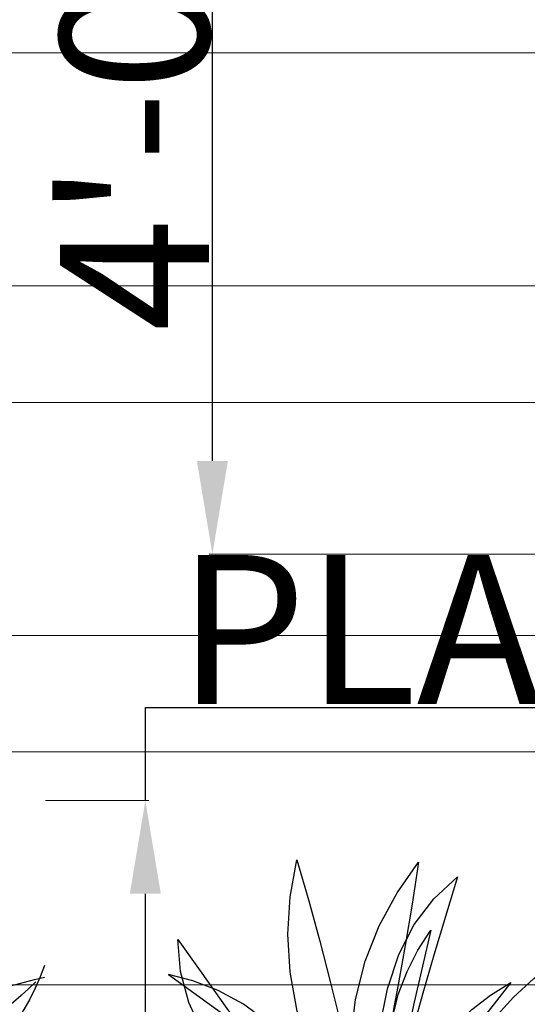
# Model space of a CAD drawing. Units: inches. Extents: x 351 to 1738, y -265 to 286.
# Tile 17 of 38: x 1209 to 1236, y -175 to -122. Entities that reach past the tile are written whole.
import ezdxf

# ---------------------------------------------------------------- set-up
doc = ezdxf.new("R2010")
doc.units = ezdxf.units.IN
doc.header["$MEASUREMENT"] = 0
doc.layers.add('A-ANNO-DIMS', color=2, linetype='Continuous', lineweight=18)
doc.layers.add('A-FLOR-PATT', color=9, linetype='Continuous', lineweight=9)
for name, color, linetype in [('CAY', 94, 'Continuous'), ('CHITIET', 144, 'Continuous'), ('DIENHOA', 3, 'Continuous'), ('netmanh', 9, 'Continuous'), ('VATDUNG', 9, 'Continuous')]:
    doc.layers.add(name, color=color, linetype=linetype)
doc.styles.get("Standard").update_dxf_attribs({"font": 'arial.ttf'})
doc.dimstyles.get("Standard").update_dxf_attribs({"dimtxt": 8, "dimasz": 5, "dimexe": 0.18, "dimexo": 0.0625, "dimgap": 0.09, "dimtad": 1, "dimtoh": 1, "dimzin": 0, "dimdsep": 46, "dimlunit": 4, "dimtxsty": 'Standard', "dimcen": 0, "dimclre": 256, "dimadec": 0, "dimazin": 0, "dimtfac": 1, "dimtofl": 0, "dimtmove": 0, "dimatfit": 3, "dimfxl": 1, "dimtolj": 1, "dimtzin": 0, "dimlwe": -1, "dimarcsym": 0})

# ---------------------------------------------------------------- blocks, each defined once
blk = doc.blocks.new('Cay03_mb')
at = {"layer": 'DIENHOA'}
for p, q in [((118.6, 555.3), (166.2, 599.1)), ((166.2, 599.1), (142.2, 519.4)), ((79.5, 503.7), (118.6, 555.3)), ((142.2, 519.4), (119, 441.7)), ((48.6, 443.6), (79.5, 503.7)), ((25.5, 374.3), (48.6, 443.6)), ((119, 441.7), (96.7, 365.6)), ((-365.2, 390.3), (-414.4, 402.8)), ((-414.4, 402.8), (-240.2, 277.8)), ((-314.9, 371.3), (-365.2, 390.3)), ((-263.5, 343.5), (-314.9, 371.3)), ((9.9, 295.3), (25.5, 374.3)), ((96.7, 365.6), (75.6, 290.6)), ((-211.2, 304.6), (-263.5, 343.5))]:
    blk.add_line(p, q, dxfattribs=at)
for points in [[(23.7, -5.4), (-41, 82.2), (-91.8, 167.1), (-129.7, 249.5), (-155.6, 329.6), (-170.2, 407.8), (-174.7, 484.2), (-169.8, 559.3), (-156.5, 633.1)], [(-156.5, 633.1), (-132.5, 551.3), (-110.5, 470), (-89.8, 389.2), (-69.6, 309), (-49, 229.4), (-27.1, 150.4), (-3.2, 72.1), (23.7, -5.4)], [(-16.4, -26.7), (-38.3, 80), (-48.9, 178.3), (-48.7, 269), (-38.5, 352.6), (-19.1, 429.7), (9, 501), (44.9, 567.1), (87.9, 628.5)], [(87.9, 628.5), (75.5, 544.2), (61.3, 461.2), (46.1, 379.1), (30.8, 297.8), (16.1, 216.9), (2.9, 136), (-8.3, 54.9), (-16.4, -26.7)], [(23.7, -5.4), (19.8, 93), (20.3, 177), (25, 248.5), (34, 309.8), (47.3, 362.7), (64.9, 409.3), (86.8, 451.7), (112.9, 491.9)], [(112.9, 491.9), (96, 419.7), (79.5, 347.4), (63.9, 276.5), (50, 208.4), (38.4, 144.8), (29.7, 86.9), (24.6, 36.3), (23.7, -5.4)], [(-395.6, 473.7), (-347.5, 405.6), (-300.6, 339.5), (-254.3, 275.1), (-208.3, 212.3), (-161.9, 150.9), (-114.8, 90.7), (-66.5, 31.6), (-16.4, -26.7)], [(-16.4, -26.7), (-108.3, 38.6), (-186.9, 101.7), (-252.4, 163.5), (-305.1, 224.4), (-345.4, 285.2), (-373.7, 346.6), (-390.4, 409.2), (-395.6, 473.7)], [(23.7, -5.4), (79.9, 91.7), (134.1, 176.2), (185.8, 248.4), (234.3, 308.7), (279, 357.3), (319.3, 394.8), (354.6, 421.4), (384.3, 437.5)], [(273.2, 387.3), (227.6, 328.8), (182.3, 270.1), (138.4, 212.3), (97.2, 156.4), (60, 103.4), (27.8, 54.6), (1.9, 10.8), (-16.4, -26.7)], [(-16.4, -26.7), (21.4, 64.2), (57, 140.3), (91.4, 203.3), (125.2, 255.1), (159.5, 297.5), (195, 332.5), (232.7, 361.8), (273.2, 387.3)]]:
    blk.add_lwpolyline(points, dxfattribs=at)
blk = doc.blocks.new('A$C5431134F')
at = {"layer": 'VATDUNG'}
for centre, radius, start, end in [((2160.8, 1662), 1245, 150.2411, 205.809), ((5177, 1582.5), 4150.3, 170.24, 186.1148), ((-65.9, 1738.8), 1267.2, 354.3326, 25.2804), ((193.1, 3473.3), 2507.8, 289.6318, 316.9416), ((2357.8, 162.2), 1629.1, 101.2486, 143.9899), ((1000.7, 2213.1), 1133.8, 274.4073, 336.4431), ((1532.8, 1250.1), 499, 101.4267, 190.9877), ((1828.1, 1082.8), 773.2, 121.9055, 175.1859), ((3715.1, 660.2), 2523.5, 154.6853, 162.4501), ((-246.7, 51.1), 1647.5, 39.15, 81.389), ((1000.7, 2213.1), 1133.8, 208.0484, 264.6491), ((1859.5, 3770.4), 2797.6, 228.5745, 252.3842), ((1101.5, 1552.5), 361.2, 169.1166, 218.9556), ((667.9, 1279.8), 349.9, 42.8374, 76.9786), ((-929.9, 388.9), 2082.1, 20.5138, 36.0242), ((1386.4, 1856.4), 738.5, 261.6389, 315.6255), ((-169.9, 6392.7), 5465.7, 286.3355, 292.415), ((1571.2, 1428.8), 356.3, 257.3557, 344.3532), ((624.5, 223.6), 940.4, 92.4374, 115.2956), ((-65.9, 1738.8), 1267.2, 330.7697, 331.9367), ((1294.4, -49.6), 1206.1, 104.1284, 160.1468), ((-2233.8, 3749.8), 4146.2, 305.4464, 320.7382), ((2052.7, 864.5), 1083.3, 166.3603, 232.9474), ((1250.8, 281.5), 836.9, 19.4342, 107.4357), ((625, 349.3), 851.8, 6.5073, 62.3609), ((-70, 1420), 1084.7, 282.2423, 341.7321), ((546.4, 1826.6), 819.5, 246.7315, 287.3971), ((248.9, 8461.8), 7388, 269.91003, 274.50199), ((3885.3, 1488.7), 2894, 188.0959, 210.7226), ((1889.6, 1210.8), 871.9, 188.5552, 241.3289), ((-527.8, -458.7), 2192.5, 24.7599, 44.6473), ((2594.9, 3037.7), 2500, 231.5416, 257.1764), ((754.1, -691.9), 1814.1, 46.1483, 80.3711), ((1738.9, 617.5), 897.6, 155.9893, 202.84), ((2946.5, 414), 2039.9, 165.0604, 184.0737), ((1214.1, 597.8), 452.1, 154.5276, 228.0163), ((-246.7, 51.1), 1647.5, 358.2222, 17.8583)]:
    blk.add_arc(centre, radius, start, end, dxfattribs=at)
blk = doc.blocks.new('A$C5A8625A6')
at = {"layer": 'CHITIET', "ltscale": 50, "xscale": -0.49, "yscale": 0.49, "zscale": 0.49, "rotation": 180}
blk.add_blockref('A$C5431134F', (0, 1120.2), dxfattribs=at)
blk = doc.blocks.new('A$C18571848')
at = {"layer": 'netmanh', "xscale": 0.5393606399999998, "yscale": 0.5393606399999998, "zscale": 0.5393606399999998}
blk.add_blockref('A$C5A8625A6', (0, 0), dxfattribs=at)
blk = doc.blocks.new('*D36')
at = {"layer": 'A-ANNO-DIMS', "transparency": 16777216}
for p, q in [((1073.569, -199.341), (1073.569, -204.202)), ((1105.198, -199.341), (1105.198, -204.202))]:
    blk.add_line(p, q, dxfattribs=at)
at = {"layer": 'A-ANNO-DIMS', "color": 0, "lineweight": -2, "transparency": 16777216}
for p, q in [((1078.569, -204.022), (1100.198, -204.022)), ((1105.198, -204.022), (1227.071, -204.022))]:
    blk.add_line(p, q, dxfattribs=at)
at = {"layer": 'A-ANNO-DIMS', "color": 0, "transparency": 16777216}
for points in [[(1078.569, -203.189), (1078.569, -204.856), (1073.569, -204.022)], [(1100.198, -203.189), (1100.198, -204.856), (1105.198, -204.022)]]:
    blk.add_solid(points, dxfattribs=at)
at = {"layer": 'Defpoints', "color": 0, "transparency": 16777216}
for p in [(1073.569, -199.278), (1105.198, -199.278), (1105.198, -204.022)]:
    blk.add_point(p, dxfattribs=at)
at = {"layer": 'A-ANNO-DIMS', "color": 0, "transparency": 16777216, "insert": (1168.634, -199.796), "char_height": 8, "attachment_point": 5}
blk.add_mtext('\\A1;PLANT A 2\'-7 1/2" TYP.', dxfattribs=at)
blk = doc.blocks.new('*D38')
at = {"layer": 'A-ANNO-DIMS', "color": 0, "lineweight": -2, "transparency": 16777216}
for p, q in [((1215.465, -164.135), (1215.465, -159.135)), ((1215.465, -159.135), (1313.607, -159.135)), ((1215.465, -195.235), (1215.465, -169.135))]:
    blk.add_line(p, q, dxfattribs=at)
at = {"layer": 'A-ANNO-DIMS', "transparency": 16777216}
for p, q in [((1210.112, -164.135), (1215.645, -164.135)), ((1210.112, -200.235), (1215.645, -200.235))]:
    blk.add_line(p, q, dxfattribs=at)
at = {"layer": 'A-ANNO-DIMS', "color": 0, "transparency": 16777216}
for points in [[(1214.631, -169.135), (1216.298, -169.135), (1215.465, -164.135)], [(1214.631, -195.235), (1216.298, -195.235), (1215.465, -200.235)]]:
    blk.add_solid(points, dxfattribs=at)
at = {"layer": 'Defpoints', "color": 0, "transparency": 16777216}
for p in [(1210.05, -164.135), (1215.465, -164.135), (1210.05, -200.235)]:
    blk.add_point(p, dxfattribs=at)
at = {"layer": 'A-ANNO-DIMS', "color": 0, "transparency": 16777216, "insert": (1264.581, -154.958), "char_height": 8, "attachment_point": 5}
blk.add_mtext('\\A1;PLANT B 3\'-0" TYP.', dxfattribs=at)
blk = doc.blocks.new('*D65')
at = {"layer": 'A-ANNO-DIMS', "transparency": 16777216}
for p, q in [((1248.45, -102.915), (1218.882, -102.915)), ((1248.45, -150.915), (1218.882, -150.915))]:
    blk.add_line(p, q, dxfattribs=at)
at = {"layer": 'A-ANNO-DIMS', "color": 0, "lineweight": -2, "transparency": 16777216}
blk.add_line((1219.062, -145.915), (1219.062, -107.915), dxfattribs=at)
at = {"layer": 'A-ANNO-DIMS', "color": 0, "transparency": 16777216}
for points in [[(1218.229, -107.915), (1219.896, -107.915), (1219.062, -102.915)], [(1218.229, -145.915), (1219.896, -145.915), (1219.062, -150.915)]]:
    blk.add_solid(points, dxfattribs=at)
at = {"layer": 'Defpoints', "color": 0, "transparency": 16777216}
for p in [(1219.062, -102.915), (1248.512, -102.915), (1248.512, -150.915)]:
    blk.add_point(p, dxfattribs=at)
at = {"layer": 'A-ANNO-DIMS', "color": 0, "transparency": 16777216, "insert": (1214.888, -126.915), "char_height": 8, "attachment_point": 5, "rotation": 90}
blk.add_mtext('\\A1;4\'-0"', dxfattribs=at)

msp = doc.modelspace()

# ---------------------------------------------------------------- hatches: boundary and pattern name
at = {"layer": 'A-FLOR-PATT', "transparency": 33554559}
h = msp.add_hatch(dxfattribs=at)
h.set_pattern_fill('ANSI37', color=256, scale=200, angle=135)
h.set_pattern_definition([(180, (1112.704, -164.037), (-2e-15, -25), []), (270, (1112.704, -164.037), (25, -5e-15), [])])
h.paths.add_polyline_path([(1380.064, 73.463), (1380.132, 148.463), (1338.064, 148.463), (1290.704, 148.463), (1290.704, 88.463), (1248.704, 88.463), (1248.704, -2.009), (1244.704, -2.009), (1244.704, 142.457), (1160.704, 142.457), (1160.704, 158.963), (1160.704, 170.137), (1160.704, 206.137), (1160.704, 228.963), (1112.704, 228.963), (1112.704, 209.963), (1112.704, 168.963), (1124.704, 168.963), (1124.704, 162.963), (1112.704, 162.963), (1112.704, 64.463), (1112.704, 60.463), (1112.704, 0.463), (1112.704, -48.026), (1146.804, -47.981), (1146.804, -35.691), (1207.804, -35.691), (1207.804, -47.902), (1236.542, -47.864), (1236.544, -50.009), (1248.5, -50.009), (1248.506, -102.915), (1248.512, -150.915), (1248.514, -164.037), (1248.549, -164.037), (1273.017, -164.037), (1273.017, -128.799), (1355.24, -128.799), (1355.24, -164.037), (1384.204, -164.037), (1384.204, -57.037), (1380.064, -57.037), (1380.064, -48.037), (1392.064, -48.037), (1392.064, -53.037), (1406.549, -53.037), (1406.549, -57.037), (1401.204, -57.037), (1401.204, -147.037), (1468.204, -147.037), (1468.204, -138.5), (1472.204, -138.5), (1472.204, -102.5), (1468.204, -102.5), (1468.204, -57.037), (1442.549, -57.037), (1442.549, -53.037), (1463.049, -53.037), (1463.049, -40.747), (1524.049, -40.747), (1524.049, -48.037), (1536.064, -48.037), (1536.064, -53.037), (1557.704, -53.037), (1557.704, 204.963), (1384.204, 204.963), (1384.204, 73.463), (1392.064, 73.463), (1392.064, 64.463), (1384.204, 64.463), (1384.204, -3.5), (1380.204, -3.537), (1380.204, 64.463), (1380.064, 64.463)])
h.paths.add_polyline_path([(1510.714, 86.458, -0.103984), (1511.661, 85.595, 0.470438), (1510.158, 87.614, 0.0961)], flags=16)
h.paths.add_polyline_path([(1510.443, 100.266, 0.009798), (1504.693, 100.48, 0.02879), (1504.6, 99.767, -0.165331), (1505.519, 96.135, -0.143601)], flags=16)
h.paths.add_polyline_path([(1487.201, 85.595, -0.103984), (1488.148, 86.458, 0.0961), (1488.704, 87.614, 0.470438)], flags=0)
h.paths.add_polyline_path([(1495.052, 100.43), (1494.178, 100.43, -0.026463), (1494.262, 99.774, -0.144219)], flags=16)
h.paths.add_polyline_path([(1444.485, 86.458, -0.103984), (1445.433, 85.595, 0.470438), (1443.93, 87.614, 0.0961)], flags=16)
h.paths.add_polyline_path([(1420.972, 85.595, -0.103984), (1421.92, 86.458, 0.0961), (1422.475, 87.614, 0.470438)], flags=16)
h.paths.add_polyline_path([(1428.632, 100.335, 0.001054), (1427.971, 100.309, -0.021524), (1428.033, 99.774, -0.114301)], flags=16)
h.paths.add_polyline_path([(1419.906, 143.708, 0.024979), (1420.222, 157.526), (1421.573, 159.101), (1421.573, 175.369), (1391.393, 175.369), (1391.393, 200.519), (1542.294, 200.519), (1542.294, 175.369), (1512.028, 175.369, 0.019865), (1511.521, 153.838, 0.025134), (1512.758, 118.323, 0.020553), (1512.942, 115.253), (1419.834, 115.253, -0.000414), (1419.843, 124.798), (1413.059, 124.798), (1413.059, 84.437, -0.061853), (1415.831, 80.45, -0.093077), (1420.972, 85.595, -0.267537), (1422.371, 84.732, 0.08511), (1424.052, 84.616, -0.885393), (1424.033, 84.851, -1.125815), (1424.073, 84.366, -0.087987), (1422.371, 84.732, -0.267537), (1422.326, 83.089, -0.370542), (1420.972, 85.595, 0.093077), (1415.831, 80.45, -0.087414), (1417.914, 73.937), (1418.941, 73.937, 0.02725), (1418.913, 76.906, -0.115703), (1421.051, 73.937), (1445.354, 73.937, -0.115703), (1447.492, 76.906, 0.02725), (1447.464, 73.937), (1448.491, 73.937, -0.087414), (1450.574, 80.45, 0.093077), (1445.433, 85.595, -0.370542), (1444.079, 83.089, -0.267537), (1444.034, 84.732, -0.087987), (1442.332, 84.366, -1.125815), (1442.372, 84.851, -2.032736), (1442.364, 84.368, 0.086378), (1444.034, 84.732, -0.267537), (1445.433, 85.595, -0.093077), (1450.574, 80.45, -0.257732), (1466.483, 90.927, -0.47867), (1468.832, 91.907, -0.47867), (1471.18, 90.927, -0.26264), (1483.053, 81.78, -0.071866), (1487.201, 85.595, -0.267537), (1488.6, 84.732, 0.08511), (1490.28, 84.616, -0.885393), (1490.262, 84.851, -1.125815), (1490.301, 84.366, -0.087987), (1488.6, 84.732, -0.267537), (1488.554, 83.089, -0.370542), (1487.201, 85.595, 0.071866), (1483.053, 81.78, -0.132065), (1484.143, 73.937), (1485.169, 73.937, 0.02725), (1485.142, 76.906, -0.115703), (1487.28, 73.937), (1511.582, 73.937, -0.115703), (1513.72, 76.906, 0.02725), (1513.693, 73.937), (1514.719, 73.937, -0.087414), (1516.802, 80.45, 0.093077), (1511.661, 85.595, -0.370542), (1510.308, 83.089, -0.267537), (1510.262, 84.732, -0.087987), (1508.561, 84.366, -1.125815), (1508.601, 84.851, -2.032736), (1508.592, 84.368, 0.086378), (1510.262, 84.732, -0.267537), (1511.661, 85.595, -0.093077), (1516.802, 80.45, -0.061853), (1519.575, 84.437), (1519.575, 73.937), (1413.059, 73.937), (1413.059, 124.798), (1419.843, 124.798, -0.000821)], flags=16)
h.paths.add_polyline_path([(1220.149, 54.133, -0.103984), (1220.869, 53.476, 0.470438), (1219.727, 55.011, 0.0961)], flags=16)
h.paths.add_polyline_path([(1219.944, 64.626, 0.009798), (1215.574, 64.789, 0.02879), (1215.503, 64.247, -0.165331), (1216.201, 61.487, -0.143601)], flags=16)
h.paths.add_polyline_path([(1209.779, 64.449, 0.097446), (1209.339, 64.751), (1208.247, 64.751, 0.12739), (1207.7, 64.326, 0.171586), (1206.95, 61.475, -0.158854), (1207.636, 59.45, 0.015898), (1207.795, 59.218, 0.061546), (1208.598, 59.616, 0.175416), (1208.638, 60.099, -0.284779), (1209.348, 62.472, 0.326216)], flags=16)
h.paths.add_polyline_path([(1169.818, 54.133, -0.103984), (1170.538, 53.476, 0.470438), (1169.396, 55.011, 0.0961)], flags=16)
h.paths.add_polyline_path([(1159.017, 62.472, 0.284764), (1158.307, 60.099, -0.175433), (1158.267, 59.616, 0.39293), (1159.448, 64.449, -0.32623)], flags=16)
h.paths.add_polyline_path([(1156.342, 58.239, -0.178321), (1154.011, 55.31, -0.174736), (1154.722, 55.233, -0.200802), (1156.27, 56.086, 0.12699), (1157.283, 58.991, -0.091205)], flags=16)
h.paths.add_polyline_path([(1156.624, 61.413, 0.157275), (1157.316, 64.247, 0.169622)], flags=16)
h.paths.add_polyline_path([(1152.67, 54.133, -0.0961), (1151.95, 53.476, 0.064076), (1154.465, 54.384, 0.199016)], flags=16)
h.paths.add_polyline_path([(1202.281, 53.476, -0.103984), (1203, 54.133, 0.0961), (1203.423, 55.011, 0.470438)], flags=0)
h.paths.add_polyline_path([(1151.139, 97.64, 0.024979), (1151.379, 108.141), (1152.406, 109.338), (1152.406, 121.701), (1129.47, 121.701), (1129.47, 140.814), (1244.149, 140.814), (1244.149, 121.701), (1221.148, 121.701, 0.019865), (1220.763, 105.338, 0.025134), (1221.703, 78.349, 0.020553), (1221.843, 76.016), (1151.078, 76.016, -0.128743), (1148.786, 65.037, 0.539352), (1150.327, 64.171, -0.027594), (1163.481, 64.751, 0.097695), (1163.04, 64.449, 0.326216), (1163.471, 62.472, -0.284777), (1164.181, 60.099, -0.194757), (1165.846, 61.443, -0.155402), (1165.172, 64.247, -0.166022), (1165.869, 61.475, -0.177014), (1167.852, 62.77, -0.448203), (1169.974, 60.807, -0.393499), (1167.679, 57.86, -0.895548), (1168.438, 54.524, -0.355767), (1166.218, 56.086, -0.066024), (1165.505, 57.539), (1165.251, 56.243, -0.371732), (1164.02, 59.758, -0.373614), (1163.04, 64.449, -0.097695), (1163.481, 64.751, 0.021354), (1153.294, 64.429, -0.134183), (1156.695, 61.368, 0.186873), (1154.636, 62.77, 0.448203), (1152.514, 60.807, 0.403726), (1154.905, 57.846, 0.711219), (1153.334, 55, 0.53154), (1151.95, 53.476, -0.267537), (1153.013, 52.821, 0.08511), (1154.29, 52.732, -0.885393), (1154.276, 52.911, -1.125815), (1154.306, 52.543, -0.087987), (1153.013, 52.821, -0.267537), (1152.978, 51.572, -0.370542), (1151.95, 53.476, 0.093077), (1148.043, 49.566, -0.087414), (1149.626, 44.617), (1150.406, 44.617, 0.02725), (1150.385, 46.873, -0.115703), (1152.01, 44.617), (1170.478, 44.617, -0.115703), (1172.103, 46.873, 0.02725), (1172.082, 44.617), (1172.862, 44.617, -0.087414), (1174.445, 49.566, 0.093077), (1170.538, 53.476, -0.370542), (1169.51, 51.572, -0.267537), (1169.475, 52.821, -0.087987), (1168.182, 52.543, -1.125815), (1168.212, 52.911, -2.032736), (1168.206, 52.544, 0.086378), (1169.475, 52.821, -0.267537), (1170.538, 53.476, -0.093077), (1174.445, 49.566, -0.257732), (1186.536, 57.528, -0.47867), (1188.321, 58.273, -0.47867), (1190.106, 57.528, -0.26264), (1199.128, 50.577, -0.071866), (1202.281, 53.476, -0.267537), (1203.344, 52.821, 0.08511), (1204.621, 52.732, -0.885393), (1204.607, 52.911, -1.125815), (1204.637, 52.543, -0.087987), (1203.344, 52.821, -0.267537), (1203.309, 51.572, -0.370542), (1202.281, 53.476, 0.071866), (1199.128, 50.577, -0.132065), (1199.957, 44.617), (1200.737, 44.617, 0.02725), (1200.716, 46.873, -0.115703), (1202.341, 44.617), (1220.809, 44.617, -0.115703), (1222.434, 46.873, 0.02725), (1222.413, 44.617), (1223.193, 44.617, -0.087414), (1224.776, 49.566, 0.093077), (1220.869, 53.476, -0.370542), (1219.841, 51.572, -0.267537), (1219.806, 52.821, -0.087987), (1218.513, 52.543, -1.125815), (1218.543, 52.911, -2.032736), (1218.537, 52.544, 0.086378), (1219.806, 52.821, -0.267537), (1220.869, 53.476, -0.093077), (1224.776, 49.566, -0.061853), (1226.883, 52.597), (1226.883, 44.617), (1145.936, 44.617), (1145.936, 83.269), (1151.091, 83.269, -0.000821)], flags=16)
h.paths.add_polyline_path([(1218.01, 57.86, -0.895548), (1218.769, 54.524, -0.355767), (1216.549, 56.086, -0.066024), (1215.836, 57.539), (1215.582, 56.243, -0.371732), (1214.351, 59.758, -0.373614), (1213.371, 64.449, 0.326216), (1213.802, 62.472, -0.284777), (1214.512, 60.099, -0.194757), (1216.177, 61.443, -0.179991), (1218.183, 62.77, -0.448203), (1220.305, 60.807, -0.393499)], flags=16)
h.paths.add_polyline_path([(1424.735, 91.363, -0.393499), (1421.715, 95.241, -0.448203), (1424.507, 97.824, -0.179991), (1427.147, 96.077, -0.194757), (1429.338, 94.309, -0.284777), (1430.272, 97.432, 0.326216), (1430.839, 100.034, -0.373614), (1429.55, 93.861, -0.371732), (1427.929, 89.235), (1427.596, 90.941, -0.066024), (1426.657, 89.029, -0.355767), (1423.736, 86.973, -0.895548)], flags=16)
h.paths.add_polyline_path([(1238.033, 131.257, -1), (1227.329, 131.257, -1)], flags=0)
h.paths.add_polyline_path([(1235.357, 131.257, -1), (1230.005, 131.257, -1)], flags=0)
h.paths.add_polyline_path([(1214.039, 54.243, 0.154382), (1214.38, 53.992, 0.358955), (1213.613, 54.016, 0.603948), (1214.379, 53.657, 0.371319), (1213.968, 52.872, 0.187994), (1214.312, 52.809, -0.592455), (1213.953, 52.967, -0.294279), (1214.083, 53.691, -1.300187), (1213.881, 54.134, -0.283762), (1214.469, 53.896, 1.15094)], flags=16)
h.paths.add_polyline_path([(1212.091, 56.286, -0.408434), (1211.337, 56.445, -0.036259), (1211.098, 56.848, -0.236098), (1211.59, 56.63, 0.035345), (1211.835, 56.543, -0.475241), (1212.091, 56.286, -0.475241), (1212.438, 56.182, 0.035345), (1212.631, 56.007, -0.236098), (1213.056, 55.676, -0.036259), (1212.588, 55.697, -0.408434)], flags=16)
h.paths.add_polyline_path([(1211.469, 50.297, 0.296043), (1210.47, 50.527, 0.310883), (1211.931, 50.148, 0.021255)], flags=16)
h.paths.add_polyline_path([(1213.739, 51.818, -0.036259), (1213.271, 51.838, -0.408434), (1212.774, 52.427, -0.094786), (1212.293, 50.703, 1.150474), (1212.911, 50.232, 0.166288), (1213.265, 50.68, -0.025254), (1212.603, 50.13, 1.087932), (1212.471, 49.407, 0.166288), (1213.02, 49.251, -0.016128), (1212.567, 49.563, -0.286859), (1212.217, 49.638, 0.022156), (1212.046, 50.055, -0.64613), (1212.185, 50.498, 0.088412), (1212.732, 52.077, -1.186037), (1213.121, 52.323, 0.035345), (1213.314, 52.148, -0.236098)], flags=16)
h.paths.add_polyline_path([(1212.094, 50.342, -0.048524), (1211.54, 49.605, -1.103834), (1211.397, 48.738, -0.785515), (1211.683, 48.254, -0.392043), (1210.948, 48.525, -0.392819), (1210.561, 47.995, -0.592455), (1210.201, 48.153, -0.294279), (1210.331, 48.877, -0.704172), (1210.316, 49.592, -0.679344), (1210.729, 50.112, 0.563676)], flags=16)
h.paths.add_polyline_path([(1211.274, 49.829, -0.139826), (1210.745, 49.859, -0.217879), (1210.948, 49.509, -0.498572)], flags=0)
h.paths.add_polyline_path([(1433.426, 81.49, -0.181571), (1434.245, 81.788, -0.008067), (1433.726, 82.205, 0.045578), (1432.755, 81.242, 0.179011)], flags=16)
h.paths.add_polyline_path([(1434.146, 81.009, -0.132442), (1433.645, 80.771, 0.259089), (1433.234, 80.471, -0.180211), (1433.392, 80.805, -0.16994), (1432.758, 81.109, 0.032652), (1433.273, 80.474, -0.493363), (1434.046, 80.146, -0.390497)], flags=16)
h.paths.add_polyline_path([(1434.83, 80.047, -0.947538), (1435.294, 79.576, -0.299128), (1434.625, 79.404, -0.270439), (1435.01, 78.591, -0.592455), (1434.537, 78.382, -0.392819), (1434.027, 79.08, -0.392043), (1433.06, 78.723, -0.352042), (1433.003, 79.197, -0.197216), (1433.75, 79.734, -0.71364), (1434.447, 79.939, -0.21479), (1434.819, 80.475, 0.408833), (1435.075, 80.803, -0.226152)], flags=16)
h.paths.add_polyline_path([(1432.67, 81.217, -0.454218), (1431.897, 79.923, -0.414411), (1431.301, 80.035, 0.016129), (1431.897, 80.445, 0.27957), (1432.073, 80.871, -0.289504), (1431.103, 81.321, -0.414411), (1430.978, 81.915, 0.01613), (1431.586, 81.521, 0.341293), (1432.125, 81.583, -0.813186)], flags=16)
h.paths.add_polyline_path([(1429.893, 86.381, -0.947538), (1430.358, 85.91, -0.173106), (1429.984, 85.712, -0.038817), (1431.625, 84.214, -0.0879), (1432.097, 88.549, -0.049768), (1431.254, 88.49, -0.236098), (1431.814, 88.925, 0.035345), (1432.067, 89.155, -0.475241), (1432.524, 89.291, -0.475241), (1432.86, 89.63, 0.035345), (1433.182, 89.744, -0.236098), (1433.83, 90.032, -0.036259), (1433.516, 89.502, -0.408434), (1432.524, 89.291, -0.312424), (1432.106, 88.58, 0.088559), (1431.625, 84.214, -0.408434), (1430.971, 83.439, -0.036259), (1430.355, 83.412, -0.236098), (1430.914, 83.847, 0.035345), (1431.168, 84.078, -0.475241), (1431.625, 84.214, 0.038817), (1429.984, 85.712, -0.321732), (1429.333, 86.048, -0.32743), (1429.883, 86.809, 0.408833), (1430.138, 87.138, -0.226152)], flags=16)
h.paths.add_polyline_path([(1211.206, 58.616, -0.999784), (1211.336, 59.323, -0.614994)], flags=16)
h.paths.add_polyline_path([(1210.288, 49.429, 0.154382), (1210.629, 49.178, 0.358955), (1209.861, 49.202, 0.603948), (1210.627, 48.843, -0.534825), (1210.806, 49.295, 0.748346)], flags=16)
h.paths.add_polyline_path([(1209.589, 51.828, -0.008791), (1209.775, 51.753, 0.112231), (1209.466, 52.019, 1.418851), (1209.014, 51.708, -0.458726), (1208.651, 51.073, -0.592455), (1208.291, 51.232, -0.294279), (1208.421, 51.955, -1.300187), (1208.219, 52.398, -0.226005), (1208.719, 52.257, -0.475519), (1209.158, 52.369, -1.455499), (1209.603, 52.664, 0.421305), (1209.191, 52.262, -0.591212), (1208.979, 51.796, 0.497399), (1209.773, 51.333, 0.649312)], flags=16)
h.paths.add_polyline_path([(1208.029, 52.041, 0.544667), (1208.832, 52.045, 0.220132)], flags=0)
h.paths.add_polyline_path([(1210.438, 51.425, -0.2042), (1210.277, 52.018, 0.270826), (1209.915, 52.897, 0.324115)], flags=0)
h.paths.add_polyline_path([(1209.668, 52.407, -0.60139), (1208.99, 52.221, -0.394916), (1208.248, 52.83, -0.836792), (1208.651, 53.017, -0.338488), (1209.039, 52.571, 0.194138), (1209.191, 52.262, 0.413995), (1209.712, 52.475, 0.51771), (1210.503, 51.416, 0.401922), (1209.493, 50.93, 0.206396), (1209.516, 50.165, -0.319463), (1210.417, 51.418, -0.466635)], flags=16)
h.paths.add_polyline_path([(1206.601, 56.086, -0.355767), (1204.381, 54.524, -0.921198), (1205.236, 57.846, 0.206569), (1207.614, 58.991, -0.12699)], flags=16)
h.paths.add_polyline_path([(1435.487, 82.816, 0.527765), (1436.615, 83.361, 0.50854), (1437.05, 82.433, 0.592455), (1437.524, 82.641, 0.331245), (1436.963, 83.548, 0.387863), (1437.808, 83.626, 0.592954), (1437.618, 84.176, 0.226016), (1436.961, 83.99, 0.318205), (1437.588, 84.854, 0.689374), (1437.05, 84.991, 0.335765), (1436.539, 84.41, -0.156993), (1436.404, 84.065, -0.434611), (1436.961, 83.99, -0.21479), (1437.333, 84.526, 0.408833), (1437.588, 84.854, -0.226152), (1437.343, 84.097, -0.947538), (1437.808, 83.626, -0.299128), (1437.139, 83.455, -0.270439), (1437.524, 82.641, -0.592455), (1437.05, 82.433, -0.392819), (1436.541, 83.13, -0.43966), (1435.475, 82.794, -0.174614), (1435.942, 82.244, -0.206396), (1435.912, 81.237, -0.270826), (1435.125, 82.208, 0.207976), (1434.686, 82.904, -0.196495)], flags=16)
h.paths.add_polyline_path([(1435.386, 84.832, 0.270811), (1434.91, 83.676, -0.204217), (1434.699, 82.895, 0.324115)], flags=0)
h.paths.add_polyline_path([(1435.68, 84.18, -0.217656), (1435.554, 83.304, -0.176705), (1436.236, 83.778, -0.373036)], flags=0)
h.paths.add_polyline_path([(1435.566, 100.034, 0.326216), (1436.133, 97.432, -0.284777), (1437.067, 94.309, -0.194757), (1439.258, 96.077, -0.155402), (1438.371, 99.767, -0.166022), (1439.289, 96.12, -0.177014), (1441.897, 97.824, -0.448203), (1444.69, 95.241, -0.393499), (1441.67, 91.363, -0.895548), (1442.669, 86.973, -0.355767), (1439.748, 89.029, -0.066024), (1438.809, 90.941), (1438.476, 89.235, -0.371732), (1436.855, 93.861, -0.373614)], flags=16)
h.paths.add_polyline_path([(1191.252, 49.507, -0.274022), (1190.658, 48.409, 0.267537), (1191.311, 47.344, 0.370542)], flags=0)
h.paths.add_polyline_path([(1190.301, 49.717, 0.199016), (1188.619, 49.04, 0.064076), (1191.252, 49.507, -0.0961)], flags=0)
h.paths.add_polyline_path([(1189.518, 47.857, 1.125815), (1189.676, 47.523, 2.044605)], flags=0)
h.paths.add_polyline_path([(1464.974, 80.372, 0.274022), (1465.756, 78.927, -0.083013)], flags=0)
h.paths.add_polyline_path([(1464.974, 80.372, 0.370542), (1464.897, 77.525, 0.576324)], flags=0)
h.paths.add_polyline_path([(1464.974, 80.372, -0.470438), (1467.284, 81.372, -0.0961), (1466.226, 80.648, -0.199016), (1468.439, 79.757, -0.064076)], flags=0)
h.paths.add_polyline_path([(1189.511, 56.43, -0.259467), (1188.321, 56.391, -0.259467), (1187.13, 56.43, 0.08511), (1188.193, 55.716, -0.885393), (1188.27, 55.878, -1.196013), (1188.355, 55.442, 0.101459)], flags=0)
h.paths.add_polyline_path([(1188.321, 57.596, 0.078072), (1187.678, 57.24, 0.01555), (1188.321, 57.136, 0.01555), (1188.964, 57.24, 0.078072)], flags=0)
h.paths.add_polyline_path([(1190.164, 55.365, -0.576324), (1190.106, 57.528, -0.198294), (1188.321, 58.319, -0.198294), (1186.536, 57.528, -0.576324), (1186.477, 55.365, -0.370542), (1186.536, 57.528, 0.198294), (1188.321, 58.319, 0.198294), (1190.106, 57.528, -0.370542)], flags=0)
h.paths.add_polyline_path([(1188.372, 55.878, 1.125814), (1188.529, 55.544, 2.044605)], flags=0)
h.paths.add_polyline_path([(1186.341, 49.717, -0.0961), (1185.389, 49.507, 0.064076), (1188.022, 49.04, 0.199016)], flags=0)
h.paths.add_polyline_path([(1185.389, 49.507, -0.267537), (1185.984, 48.409, 0.08511), (1187.046, 47.695, -0.885393), (1187.123, 47.857, -1.125815), (1186.966, 47.523, -0.087987), (1185.984, 48.409, -0.267537), (1185.331, 47.344, -0.370542)], flags=0)
h.paths.add_polyline_path([(1399.441, 187.944, -1), (1413.525, 187.944, -1)], flags=0)
h.paths.add_polyline_path([(1402.962, 187.944, -1), (1410.004, 187.944, -1)], flags=0)
h.paths.add_polyline_path([(1357.663, -72.245), (1377.272, -72.245), (1377.272, -91.854), (1357.663, -91.854)], flags=16)
h.paths.add_polyline_path([(1467.256, 78.201, -1.125815), (1467.049, 77.761, -2.044605)], flags=0)
h.paths.add_polyline_path([(1468.822, 88.714, 0.941125), (1469.106, 88.316, 1.137152), (1468.765, 88.755, 0.890986), (1468.99, 88.245, 0.094828), (1470.398, 89.481, -0.267537), (1471.18, 90.927, -0.028123), (1469.678, 90.547, -0.028774), (1469.948, 90.311, -0.020327), (1468.832, 90.41, -0.020327), (1467.716, 90.311, -0.028774), (1467.986, 90.547, -0.028123), (1466.483, 90.927, -0.267537), (1467.265, 89.481, 0.08511), (1468.663, 88.542, -1.202316)], flags=0)
h.paths.add_polyline_path([(1178.25, 124.523, -0.119929), (1165.65, 124.145, -0.107349), (1159.133, 124.446, -0.102891), (1159.132, 130.465, -0.074897), (1158.993, 137.956, 0.002027), (1167.844, 137.479, -0.07553), (1180.337, 137.666, -0.075861), (1186.502, 137.688, -0.14099), (1186.272, 130.046, -0.095481), (1186.729, 124.748, -0.10603)], flags=0)
h.paths.add_polyline_path([(1469.225, 79.757, -0.199016), (1471.437, 80.648, -0.0961), (1470.379, 81.372, -0.470438), (1472.689, 80.372, -0.370542), (1472.766, 77.525, -0.267537), (1471.907, 78.927, -0.087986), (1470.615, 77.761, -1.125849), (1470.408, 78.201, -2.032736), (1470.642, 77.778, 0.086378), (1471.907, 78.927, -0.267537), (1472.689, 80.372, -0.064076)], flags=0)
h.paths.add_polyline_path([(1430.423, 186.902, -0.074897), (1430.24, 196.758, 0.002027), (1441.887, 196.131, -0.07553), (1458.326, 196.377, -0.075861), (1466.438, 196.406, -0.14099), (1466.136, 186.35, -0.095481), (1466.737, 179.378, -0.10603), (1455.58, 179.082, -0.119929), (1439, 178.585, -0.107349), (1430.425, 178.981, -0.102891)], flags=0)
h.paths.add_polyline_path([(1162.258, 49.939, 0.335765), (1161.87, 49.497, -0.156994), (1161.767, 49.235, -0.434611), (1162.19, 49.178, -0.21479), (1162.473, 49.585, 1.529195)], flags=16)
h.paths.add_polyline_path([(1161.683, 49.021, 0.581518), (1161.268, 49.583, 0.592761)], flags=16)
h.paths.add_polyline_path([(1162.602, 48.058, 0.371319), (1162.192, 48.843, 0.434533), (1162.88, 48.962, 0.185081), (1162.197, 48.926, 1.121837)], flags=16)
h.paths.add_polyline_path([(1161.443, 48.941, -1.307104), (1161.495, 48.571, -0.217752), (1161.136, 48.254, 0.697303), (1161.871, 49.048, 0.121514)], flags=16)
h.paths.add_polyline_path([(1162.531, 49.429, -0.207084), (1162.05, 49.146, -0.99203)], flags=16)
h.paths.add_polyline_path([(1161.304, 49.578, -0.719667), (1161.513, 50.079, -0.130428), (1160.836, 50.168, 0.039593)], flags=0)
h.paths.add_polyline_path([(1162.036, 50.584, -0.008067), (1161.642, 50.9, 0.029367), (1161.35, 50.297, -0.205788)], flags=16)
h.paths.add_polyline_path([(1162.882, 51.392, -0.124733), (1162.763, 51.828, -0.101191), (1162.399, 51.438, -0.153425)], flags=0)
h.paths.add_polyline_path([(1164.235, 51.85, -0.309107), (1164.513, 51.136, -0.627125), (1163.781, 51.603, -0.685909), (1162.777, 51.219, -0.233285), (1163.303, 50.165, -0.270826), (1162.705, 50.903, 0.2042), (1162.381, 51.425, 0.204182), (1162.542, 52.018, -0.270841), (1162.903, 52.897, -0.127261), (1163.219, 52.529, -1.168681), (1163.781, 52.587, -0.329112), (1164.168, 53.017, -0.836792), (1164.571, 52.83, -0.193341), (1164.391, 52.338, -0.947538), (1164.744, 51.981, -0.299128)], flags=16)
h.paths.add_polyline_path([(1163.598, 51.937, -1.262956), (1163.236, 51.831, 0.012575), (1162.971, 51.721, 0.230657), (1163.151, 52.407, -0.164898), (1163.178, 52.661, -0.44932), (1163.628, 52.262, -0.721477), (1164.154, 52.088, -0.849998)], flags=0)
h.paths.add_polyline_path([(1161.613, 58.616, -0.980413), (1161.525, 59.049, -2.908935)], flags=16)
h.paths.add_polyline_path([(1160.252, 49.166, -0.414411), (1159.799, 49.251, 0.016129), (1160.252, 49.563, 0.27957), (1160.386, 49.887, -0.289504), (1159.649, 50.229, -0.414411), (1159.554, 50.68, 0.01613), (1160.015, 50.381, 0.617885), (1160.526, 50.703, -0.094786), (1160.045, 52.427, -0.140444), (1159.682, 52.042, -0.057856), (1159.3, 51.872, 0.544843), (1160.046, 52.419, -0.088122), (1160.404, 55.721, -0.049768), (1159.763, 55.676, -0.236098), (1160.188, 56.007, 0.035345), (1160.381, 56.182, -0.475241), (1160.728, 56.286, -0.475241), (1160.984, 56.543, 0.035345), (1161.229, 56.63, -0.236098), (1161.721, 56.848, -0.036259), (1161.482, 56.445, -0.408434), (1160.728, 56.286, -0.312424), (1160.411, 55.745, 0.088559), (1160.045, 52.427, 0.107081), (1160.634, 50.498, -0.494798), (1160.839, 50.149, -0.454218)], flags=16)
h.paths.add_polyline_path([(1160.666, 49.808, -2.076528), (1160.828, 50.172, 0.019586)], flags=0)
h.paths.add_polyline_path([(1158.439, 53.992, 0.154382), (1158.78, 54.243, 0.748346), (1158.262, 54.109, -0.338225), (1158.492, 53.839, -0.170816), (1159.124, 53.779, 0.495729), (1158.938, 54.134, 0.226016)], flags=16)
h.paths.add_polyline_path([(1160.045, 52.427, 0.038817), (1158.798, 53.565, -0.119818), (1158.574, 53.586, -0.309107), (1158.851, 52.872, -0.187994), (1158.506, 52.809, 0.592455), (1158.866, 52.967, 0.331245), (1158.44, 53.657, 0.201245), (1158.798, 53.565, -0.034023), (1159.901, 52.578, -0.044253), (1159.698, 52.323, -0.475241)], flags=16)
h.paths.add_polyline_path([(1336.926, -95.392), (1336.926, -117.945), (1291.82, -117.945), (1291.82, -95.392)], flags=16)
h.paths.add_polyline_path([(1357.535, -97.244), (1357.726, -96.697, 0.034844)], flags=16)
h.paths.add_polyline_path([(1376.693, -96.478), (1377.301, -96.5, 0.031497), (1375.907, -96.424), (1357.726, -96.424)], flags=16)
h.paths.add_polyline_path([(1379.403, -119.667, 0.026706), (1380.043, -119.439, -0.015299)], flags=16)
h.paths.add_polyline_path([(1357.726, -120.202), (1357.821, -120.202), (1357.821, -120.201)], flags=16)
h.paths.add_polyline_path([(1354.171, -104.592), (1354.469, -98.672, 0.011138)], flags=16)
h.paths.add_polyline_path([(1355.058, -119.136), (1354.578, -118.539, 0.143164)], flags=16)
h.paths.add_polyline_path([(1378.851, -96.821), (1378.85, -96.82), (1378.85, -96.82, -0.04968), (1380.055, -97.191), (1378.85, -96.82, 0.150054), (1375.135, -97.188), (1375.136, -119.44, -0.00997), (1374.747, -116.649), (1357.726, -116.649, 0.169385), (1357.535, -119.382), (1357.535, -119.382), (1357.535, -119.382, 0.034818), (1357.726, -119.928), (1357.726, -119.928), (1357.726, -119.929, -0.034877), (1357.535, -119.382), (1355.507, -119.382), (1355.317, -119.278), (1357.535, -119.382, -0.169394), (1357.726, -116.649, -0.039151), (1374.686, -116.113, -0.002015), (1374.625, -115.546, 0.115322), (1369.915, -115.474, 0.060921), (1369.922, -101.154, 0.115146), (1374.625, -101.079, -0.002016), (1374.686, -100.513, -0.039151), (1357.726, -99.977), (1374.747, -99.977, -0.009963), (1375.135, -97.188), (1375.135, -97.188, -0.150108)], flags=16)
h.paths.add_polyline_path([(1490.963, 91.363, -0.393499), (1487.944, 95.241, -0.448203), (1490.736, 97.824, -0.179991), (1493.376, 96.077, -0.194757), (1495.567, 94.309, -0.284777), (1496.501, 97.432, 0.326216), (1497.068, 100.034, -0.373614), (1495.778, 93.861, -0.371732), (1494.158, 89.235), (1493.824, 90.941, -0.066024), (1492.886, 89.029, -0.355767), (1489.964, 86.973, -0.895548)], flags=16)
h.paths.add_polyline_path([(1354.86, -97.658), (1355.316, -97.348, 0.101911)], flags=16)
h.paths.add_polyline_path([(1497.063, 83.327, 0.176724), (1496.37, 83.785, -0.405139), (1496.016, 83.384, 0.497399), (1497.06, 82.774, 0.649312), (1496.818, 83.426, -0.008791)], flags=16)
h.paths.add_polyline_path([(1496.339, 83.783, 0.592761), (1496.886, 84.522, 0.581518)], flags=16)
h.paths.add_polyline_path([(1495.11, 82.641, 0.592455), (1495.583, 82.433, 0.676915), (1495.805, 83.59, 0.375669)], flags=16)
h.paths.add_polyline_path([(1495.015, 84.176, -0.145057), (1495.301, 84.526, -0.408833), (1495.045, 84.854, 0.220629), (1495.381, 84.152, -0.199594), (1495.851, 83.764, -0.524017), (1494.826, 83.626, -0.592998)], flags=16)
h.paths.add_polyline_path([(1501.655, 81.915, -0.016129), (1501.048, 81.521, -0.392719), (1500.462, 81.37, -0.21067), (1500.607, 81.142, 0.306699)], flags=16)
h.paths.add_polyline_path([(1500.11, 89.291, -0.408434), (1499.118, 89.502, -0.036259), (1498.803, 90.032, -0.236098), (1499.451, 89.744, 0.035345), (1499.774, 89.63, -0.475241), (1500.11, 89.291, -0.475241), (1500.567, 89.155, 0.035345), (1500.82, 88.925, -0.236098), (1501.379, 88.49, -0.036259), (1500.763, 88.516, -0.408434)], flags=16)
h.paths.add_polyline_path([(1498.908, 82.205, -0.051322), (1500.013, 81.134, -0.587931), (1500.234, 81.676, 0.107081), (1501.009, 84.214, -0.03529)], flags=16)
h.paths.add_polyline_path([(1496.93, 83.875, -0.206396), (1497.247, 84.832, -0.270826), (1497.724, 83.676, 0.207976), (1497.944, 82.884, -0.381455)], flags=16)
h.paths.add_polyline_path([(1496.721, 81.237, 0.270812), (1497.509, 82.208, -0.204216), (1497.935, 82.895, 0.324115)], flags=16)
h.paths.add_polyline_path([(1497.529, 80.125, -0.145057), (1497.814, 80.475, -0.703182), (1498.282, 81.178, -0.122925), (1497.977, 81.714, -0.270837), (1499.207, 81.49, 0.207964), (1499.993, 81.248, -0.265145), (1499.278, 80.472, 0.381901), (1498.808, 79.947, -0.305905), (1498.848, 79.519, 0.499482), (1498.574, 79.217, -0.458726), (1498.097, 78.382, -0.592455), (1497.624, 78.591, -0.270439), (1498.009, 79.404, -0.299116), (1497.34, 79.576, -0.593016)], flags=16)
h.paths.add_polyline_path([(1500.736, 79.923, 0.414411), (1501.333, 80.035, -0.321648), (1500.192, 80.765, 0.019886), (1499.976, 81.251, 0.465331)], flags=16)
h.paths.add_polyline_path([(1501.009, 84.214, -0.038817), (1502.649, 85.712, -0.173095), (1502.276, 85.91, -0.593016), (1502.465, 86.46, -0.145057), (1502.751, 86.809, -0.408833), (1502.495, 87.138, 0.220629), (1502.831, 86.436, -0.199594), (1503.301, 86.048, -0.321732), (1502.649, 85.712, 0.038817), (1501.009, 84.214, 0.122449), (1501.412, 83.755, 0.475491), (1501.335, 84.226, 0.055822), (1501.719, 83.847, -0.236098), (1502.278, 83.412, -0.036259), (1501.663, 83.439, -0.408434)], flags=16)
h.paths.add_polyline_path([(1501.794, 100.034, 0.326216), (1502.362, 97.432, -0.284777), (1503.295, 94.309, -0.194757), (1505.486, 96.077, -0.179991), (1508.126, 97.824, -0.448203), (1510.918, 95.241, -0.393499), (1507.899, 91.363, -0.895548), (1508.898, 86.973, -0.355767), (1505.976, 89.029, -0.066024), (1505.038, 90.941), (1504.704, 89.235, -0.371732), (1503.084, 93.861, -0.373614)], flags=16)
h.paths.add_polyline_path([(1146.29, 131.257, -1), (1135.587, 131.257, -1)], flags=0)
h.paths.add_polyline_path([(1143.614, 131.257, -1), (1138.262, 131.257, -1)], flags=0)
h.paths.add_polyline_path([(1524.064, 73.463), (1536.064, 73.463), (1536.064, 64.463), (1524.064, 64.463)], flags=16)
h.paths.add_polyline_path([(1520.162, 187.944, -1), (1534.246, 187.944, -1)], flags=0)
h.paths.add_polyline_path([(1530.725, 187.944), (1527.204, 187.944), (1527.204, 184.423, 0.414214)], flags=0)
h.paths.add_polyline_path([(1278.415, -91.154), (1331.067, -91.154), (1331.067, -80.583), (1278.415, -80.583)], flags=24)
h.paths.add_polyline_path([(1266.655, -79.354), (1354.738, -79.354), (1354.738, -67.817), (1266.655, -67.817)], flags=24)
h.paths.add_polyline_path([(1115.482, 206.184), (1155.098, 206.184), (1155.098, 217.714), (1115.482, 217.714)], flags=24)
h.paths.add_polyline_path([(1161.771, 8.501), (1222.466, 8.501), (1222.466, 19.079), (1161.771, 19.079)], flags=24)
h.paths.add_polyline_path([(1164.656, 18.795), (1210.615, 18.795), (1210.615, 30.324), (1164.656, 30.324)], flags=24)
h.paths.add_polyline_path([(1368.147, -32.882), (1379.362, -32.882), (1379.362, -21.733), (1368.147, -21.733)], flags=24)
h.paths.add_polyline_path([(1244.842, -31.012), (1256.057, -31.012), (1256.057, -19.863), (1244.842, -19.863)], flags=24)
h.paths.add_polyline_path([(1114.589, 195.739), (1156.517, 195.739), (1156.517, 206.31), (1114.589, 206.31)], flags=24)
h.paths.add_polyline_path([(1436.398, 37.632), (1505.131, 37.632), (1505.131, 48.203), (1436.398, 48.203)], flags=24)
h.paths.add_polyline_path([(1435.991, 47.919), (1507.906, 47.919), (1507.906, 59.456), (1435.991, 59.456)], flags=24)
h.paths.add_polyline_path([(1415.107, -124.896), (1457.038, -124.896), (1457.038, -114.318), (1415.107, -114.318)], flags=24)
h.paths.add_polyline_path([(1417.992, -114.602), (1457.609, -114.602), (1457.609, -103.073), (1417.992, -103.073)], flags=24)
h = msp.add_hatch(dxfattribs=at)
h.set_pattern_fill('ANSI32', color=256, scale=50, angle=135)
h.set_pattern_definition([(180, (1038.704, -199.037), (-2e-15, -18.75), []), (180, (1032.454, -192.787), (-2e-15, -18.75), [])])
h.paths.add_polyline_path([(1248.506, -102.915), (1236.559, -102.916), (1236.553, -56.864), (1112.704, -57.026), (1112.704, -57.037), (1103.704, -57.037), (1103.704, -45.037), (1103.704, 98.963), (1076.434, 98.963), (1076.549, -81.037), (1071.549, -81.037), (1043.704, -81.037), (1038.704, -81.037), (1038.704, -161.037), (1043.704, -161.037), (1043.704, -173.037), (1038.704, -173.037), (1038.704, -199.037), (1562.704, -199.037), (1562.704, -173.037), (1236.549, -173.037), (1236.549, -164.037), (1236.693, -164.037), (1236.676, -150.916), (1248.512, -150.915)])
h.paths.add_polyline_path([(1236.133, -134.078), (1247.348, -134.078), (1247.348, -122.929), (1236.133, -122.929)], flags=24)
h.paths.add_polyline_path([(1308.144, -185.548), (1321.66, -185.548), (1321.66, -174.4), (1308.144, -174.4)], flags=24)
h.paths.add_polyline_path([(1121.632, -122.88), (1179.647, -122.88), (1179.647, -112.309), (1121.632, -112.309)], flags=24)
h.paths.add_polyline_path([(1124.515, -112.593), (1177.986, -112.593), (1177.986, -101.056), (1124.515, -101.056)], flags=24)
h.paths.add_polyline_path([(1091.374, 23.58), (1104.89, 23.58), (1104.89, 34.728), (1091.374, 34.728)], flags=24)

# ---------------------------------------------------------------- block references
at = {"layer": 'CAY'}
for name, p, xscale, yscale, zscale in [('A$C18571848', (1177.835, -200.235), 0.0597507335965459, 0.0597507335965459, 0.0597507335965459), ('Cay03_mb', (1227.774, -184.232), 0.0267074520028285, 0.0267074520028285, 0.0267074520028285)]:
    msp.add_blockref(name, p, dxfattribs=dict(at, xscale=xscale, yscale=yscale, zscale=zscale))

# ---------------------------------------------------------------- dimensions: what is measured, and where the dimension line sits
at = {"layer": 'A-ANNO-DIMS'}
dim = msp.add_linear_dim(base=(1219.062, -102.915), p1=(1248.512, -150.915), p2=(1248.512, -102.915), angle=90, dimstyle='Standard', override={"dimdec": 1, "dimlfac": 1, "dimrnd": 0, "dimzin": 1, "dimdsep": 46, "dimlunit": 4, "dimfrac": 2}, dxfattribs=at)
dim.commit()
dim.dimension.update_dxf_attribs({"geometry": '*D65', "text_midpoint": (1214.888, -126.915)})
dim = msp.add_linear_dim(base=(1215.465, -164.135), p1=(1210.05, -200.235), p2=(1210.05, -164.135), angle=90, text='PLANT B <> TYP.', dimstyle='Standard', override={"dimdec": 1, "dimlfac": 1, "dimrnd": 0, "dimzin": 1, "dimdsep": 46, "dimlunit": 4, "dimfrac": 2}, dxfattribs=at)
dim.commit()
dim.dimension.update_dxf_attribs({"geometry": '*D38', "text_midpoint": (1264.581, -154.958)})
dim = msp.add_linear_dim(base=(1105.198, -204.022), p1=(1073.569, -199.278), p2=(1105.198, -199.278), text='PLANT A <> TYP.', dimstyle='Standard', override={"dimdec": 1, "dimlfac": 1, "dimrnd": 0, "dimzin": 1, "dimdsep": 46, "dimlunit": 4, "dimfrac": 2}, dxfattribs=at)
dim.commit()
dim.dimension.update_dxf_attribs({"geometry": '*D36', "text_midpoint": (1168.634, -199.796)})

doc.saveas('drawing.dxf')
